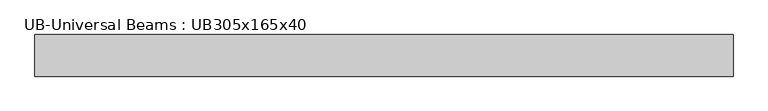
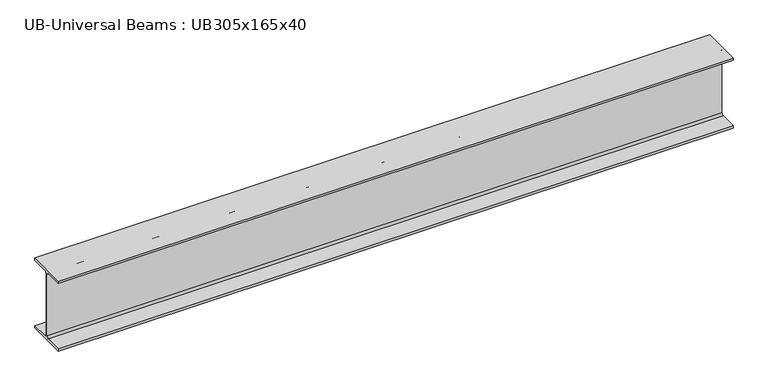
"""IFC4 building model written with IfcOpenShell, lengths in millimetres: beam geometry, UB-Universal Beams : UB305x165x40."""

from ifc_helpers import new_model, si_unit, point, frame, frame_2d, origin, place, context, project, spatial, polyline, circle_curve, trimmed, segment, composite_curve, outline, extrude, source, transform, mapped, element, save


def ub_universal_beams_ub305x165x40_9ee690e8(model_context):
    return source(origin(), model_context, "Body", "SweptSolid", [
        extrude(outline(composite_curve([segment(polyline([(82.5, -141.5), (82.5, -151.7), (-82.5, -151.7), (-82.5, -141.5), (-11.9, -141.5)]), True, "CONTINUOUS"), segment(trimmed(circle_curve(frame_2d((-11.9, -132.6)), 8.9), [point((-11.9, -141.5))], [point((-3.0, -132.6))], True, "CARTESIAN"), True, "CONTINUOUS"), segment(polyline([(-3.0, -132.6), (-3.0, 132.6)]), True, "CONTINUOUS"), segment(trimmed(circle_curve(frame_2d((-11.9, 132.6)), 8.9), [point((-3.0, 132.6))], [point((-11.9, 141.5))], True, "CARTESIAN"), True, "CONTINUOUS"), segment(polyline([(-11.9, 141.5), (-82.5, 141.5), (-82.5, 151.7), (82.5, 151.7), (82.5, 141.5), (11.9, 141.5)]), True, "CONTINUOUS"), segment(trimmed(circle_curve(frame_2d((11.9, 132.6)), 8.9), [point((11.9, 141.5))], [point((3.0, 132.6))], True, "CARTESIAN"), True, "CONTINUOUS"), segment(polyline([(3.0, 132.6), (3.0, -132.6)]), True, "CONTINUOUS"), segment(trimmed(circle_curve(frame_2d((11.9, -132.6)), 8.9), [point((3.0, -132.6))], [point((11.9, -141.5))], True, "CARTESIAN"), True, "CONTINUOUS"), segment(polyline([(11.9, -141.5), (82.5, -141.5)]), True, "CONTINUOUS")], self_intersect=False)), frame((-1325.55, 0.0, 0.0), z_axis=(1.0, 0.0, 0.0), x_axis=(0.0, 1.0, 0.0)), (0.0, 0.0, 1.0), 2765.0),
    ])


if __name__ == "__main__":
    model = new_model("IFC4")
    model_context = context("Model", 3, world=origin())
    ifc_project = project(units=[si_unit("LENGTHUNIT", "METRE", prefix="MILLI")], contexts=[model_context])
    site = spatial("IfcSite", under=ifc_project)
    building = spatial("IfcBuilding", under=site)
    placement = place(None, origin())
    ub_universal_beams_ub305x165x40_shape = ub_universal_beams_ub305x165x40_9ee690e8(model_context)
    element("IfcBeam", 1, ObjectType="UB-Universal Beams : UB305x165x40", at=placement, inside=building, context=model_context, shape_type="MappedRepresentation", body=[
        mapped(ub_universal_beams_ub305x165x40_shape, transform((0.0, 0.0, 0.0), x_axis=(1.0, 0.0, 0.0), y_axis=(0.0, 1.0, 0.0), z_axis=(0.0, 0.0, 1.0))),
    ])
    save(model, "model.ifc")

# Revit data of these elements
# Type "UB-Universal Beams : UB305x165x40"
#   Section Name Key = "UB305X165X40"
#   Width = 16.5 cm
#   Web Thickness = 0.6 cm
#   Web Fillet = 0.89 cm
#   Warping Constant = 164000.0 cm⁶
#   Torsional Moment of Inertia = 14.70 cm⁴
#   Section Area = 51.3 cm²
#   Plastic Modulus weak axis = 142.0 cm³
#   Plastic Modulus strong axis = 623.0 cm³
#   Nominal Weight = 40.2999 kgf/m
#   Moment of Inertia weak axis = 764.00 cm⁴
#   Moment of Inertia strong axis = 8503.00 cm⁴
#   Height = 30.34 cm
#   Flange Thickness = 1.02 cm
#   Elastic Modulus weak axis = 92.6 cm³
#   Elastic Modulus strong axis = 560.0 cm³
#   Centroid Vertical = 15.17 cm
#   Centroid Horizontal = 8.25 cm
#   Bolt Spacing = 9.0 cm
#   Length [instance default] = 1500 mm
#   Structural Material [instance default] = Metal - Steel 43-275
#   Type Comments = ""
#   Assembly Code = ""
# Element 1 (IfcBeam, "UB-Universal Beams : UB305x165x40")
#   Materials on its faces: "Metal - Steel 43-275"
# Materials
#   "Metal - Steel 43-275": class "Metal", colour RGB 247 247 247, transparency 0, Cost = 0
